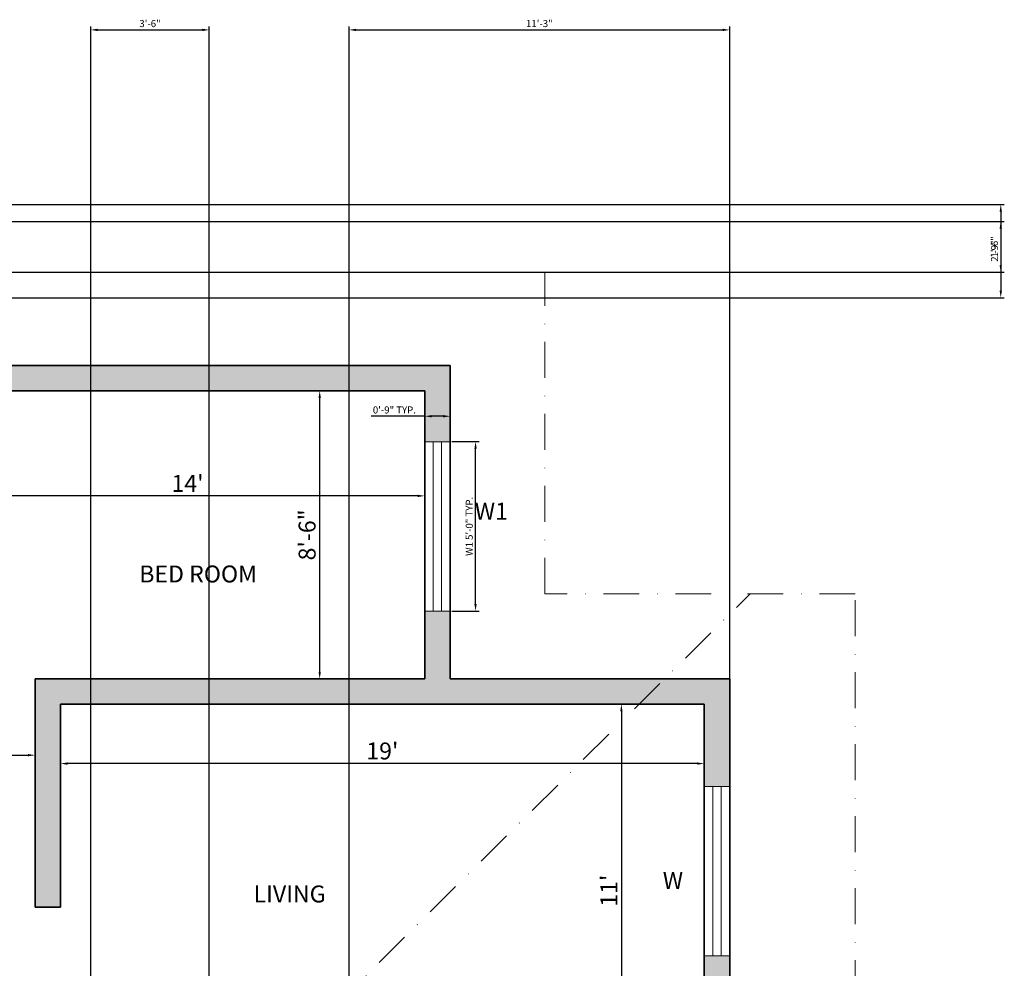
# Model space of a CAD drawing. Units: inches. Extents: x 4701 to 5398, y 2331 to 3130.
# Tile 3 of 3: x 5050 to 5398, y 2792 to 3128. Entities that reach past the tile are written whole.
import ezdxf

# ---------------------------------------------------------------- set-up
doc = ezdxf.new("R2010")
doc.units = ezdxf.units.IN
doc.linetypes.add('DASHDOT', pattern=[25.4, 12.7, -6.35, 0, -6.35])
for name, color, linetype, lineweight, true_color in [('A-ANNO-DIMS', 217, 'Continuous', 18, 0x93278f), ('A-GLAZ', 41, 'Continuous', 18, 0xf4ee51), ('A-WALL-PATT', 143, 'Continuous', 13, 0x7aafdf)]:
    doc.layers.add(name, color=color, linetype=linetype, lineweight=lineweight, true_color=true_color)
for name, color, linetype, lineweight in [('A-ANNO-TEXT', 7, 'Continuous', 18), ('A-AREA-IDEN', 7, 'Continuous', 25), ('A-ROOF-OVHD', 8, 'DASHDOT', 13), ('A-WALL', 7, 'Continuous', 35)]:
    doc.layers.add(name, color=color, linetype=linetype, lineweight=lineweight)
doc.styles.get("Standard").update_dxf_attribs({"font": 'arial.ttf'})
doc.dimstyles.new('ISO-25', dxfattribs={"dimtxt": 2.5, "dimasz": 2.5, "dimexe": 1.25, "dimexo": 0.625, "dimtad": 1, "dimlunit": 3, "dimtxsty": 'Standard', "dimcen": 2.5, "dimadec": 0, "dimazin": 0, "dimtfac": 1, "dimtmove": 0, "dimatfit": 3, "dimfxl": 1, "dimarcsym": 0})

# ---------------------------------------------------------------- blocks, each defined once
blk = doc.blocks.new('*D9')
at = {"layer": 'A-ANNO-DIMS', "color": 0, "lineweight": -2, "transparency": 16777216}
for p, q in [((5025.11, 2959.48), (5025.11, 2960.11)), ((5190.61, 2958.86), (5027.61, 2958.86)), ((5193.11, 2959.48), (5193.11, 2960.11))]:
    blk.add_line(p, q, dxfattribs=at)
at = {"layer": 'A-ANNO-DIMS', "color": 0, "transparency": 16777216}
for points in [[(5027.61, 2959.28), (5027.61, 2958.44), (5025.11, 2958.86)], [(5190.61, 2959.28), (5190.61, 2958.44), (5193.11, 2958.86)]]:
    blk.add_solid(points, dxfattribs=at)
at = {"layer": 'Defpoints', "color": 0, "transparency": 16777216}
for p in [(5025.11, 2958.86), (5025.11, 2958.86), (5193.11, 2958.86)]:
    blk.add_point(p, dxfattribs=at)
at = {"layer": 'A-ANNO-DIMS', "color": 0, "transparency": 16777216, "insert": (5109.11, 2962.5), "char_height": 6, "attachment_point": 5}
blk.add_mtext("14'", dxfattribs=at)
blk = doc.blocks.new('*D10')
at = {"layer": 'A-ANNO-DIMS', "color": 0, "lineweight": -2, "transparency": 16777216}
for p, q in [((5156.54, 2996.05), (5154.66, 2996.05)), ((5155.91, 2896.55), (5155.91, 2993.55)), ((5155.29, 2894.05), (5154.66, 2894.05))]:
    blk.add_line(p, q, dxfattribs=at)
at = {"layer": 'A-ANNO-DIMS', "color": 0, "transparency": 16777216}
for points in [[(5155.5, 2993.55), (5156.33, 2993.55), (5155.91, 2996.05)], [(5155.5, 2896.55), (5156.33, 2896.55), (5155.91, 2894.05)]]:
    blk.add_solid(points, dxfattribs=at)
at = {"layer": 'Defpoints', "color": 0, "transparency": 16777216}
for p in [(5155.91, 2996.05), (5157.16, 2996.05), (5155.91, 2894.05)]:
    blk.add_point(p, dxfattribs=at)
at = {"layer": 'A-ANNO-DIMS', "color": 0, "transparency": 16777216, "insert": (5152.23, 2945.05), "char_height": 6, "attachment_point": 5, "rotation": 90}
blk.add_mtext('8\'-6"', dxfattribs=at)
blk = doc.blocks.new('*D11')
at = {"layer": 'A-ANNO-DIMS', "color": 0, "lineweight": -2, "transparency": 16777216}
for p, q in [((5064.11, 2864.69), (5064.11, 2865.31)), ((5289.61, 2864.06), (5066.61, 2864.06)), ((5292.11, 2864.69), (5292.11, 2865.31))]:
    blk.add_line(p, q, dxfattribs=at)
at = {"layer": 'A-ANNO-DIMS', "color": 0, "transparency": 16777216}
for points in [[(5066.61, 2864.48), (5066.61, 2863.65), (5064.11, 2864.06)], [(5289.61, 2864.48), (5289.61, 2863.65), (5292.11, 2864.06)]]:
    blk.add_solid(points, dxfattribs=at)
at = {"layer": 'Defpoints', "color": 0, "transparency": 16777216}
for p in [(5064.11, 2864.06), (5064.11, 2864.06), (5292.11, 2864.06)]:
    blk.add_point(p, dxfattribs=at)
at = {"layer": 'A-ANNO-DIMS', "color": 0, "transparency": 16777216, "insert": (5178.11, 2867.75), "char_height": 6, "attachment_point": 5}
blk.add_mtext("19'", dxfattribs=at)
blk = doc.blocks.new('*D12')
at = {"layer": 'A-ANNO-DIMS', "color": 0, "lineweight": -2, "transparency": 16777216}
for p, q in [((5263.38, 2885.05), (5264, 2885.05)), ((5262.75, 2882.55), (5262.75, 2755.55)), ((5263.38, 2753.05), (5264, 2753.05))]:
    blk.add_line(p, q, dxfattribs=at)
at = {"layer": 'A-ANNO-DIMS', "color": 0, "transparency": 16777216}
for points in [[(5262.34, 2882.55), (5263.17, 2882.55), (5262.75, 2885.05)], [(5262.34, 2755.55), (5263.17, 2755.55), (5262.75, 2753.05)]]:
    blk.add_solid(points, dxfattribs=at)
at = {"layer": 'Defpoints', "color": 0, "transparency": 16777216}
for p in [(5262.75, 2885.05), (5262.75, 2753.05), (5262.75, 2753.05)]:
    blk.add_point(p, dxfattribs=at)
at = {"layer": 'A-ANNO-DIMS', "color": 0, "transparency": 16777216, "insert": (5259.12, 2819.05), "char_height": 6, "attachment_point": 5, "rotation": 90}
blk.add_mtext("11'", dxfattribs=at)
blk = doc.blocks.new('*D29')
at = {"layer": 'A-ANNO-DIMS', "color": 0, "lineweight": -2, "transparency": 16777216}
for p, q in [((4908.5, 2867.66), (4908.5, 2868.28)), ((4911, 2867.03), (5052.61, 2867.03)), ((5055.11, 2867.66), (5055.11, 2868.28))]:
    blk.add_line(p, q, dxfattribs=at)
at = {"layer": 'A-ANNO-DIMS', "color": 0, "transparency": 16777216}
for points in [[(4911, 2867.45), (4911, 2866.62), (4908.5, 2867.03)], [(5052.61, 2867.45), (5052.61, 2866.62), (5055.11, 2867.03)]]:
    blk.add_solid(points, dxfattribs=at)
at = {"layer": 'Defpoints', "color": 0, "transparency": 16777216}
for p in [(4908.5, 2867.03), (5055.11, 2867.03), (5055.11, 2867.03)]:
    blk.add_point(p, dxfattribs=at)
at = {"layer": 'A-ANNO-DIMS', "color": 0, "transparency": 16777216, "insert": (4981.8, 2868.94), "char_height": 2.5, "attachment_point": 5}
blk.add_mtext('12\'-2.61"', dxfattribs=at)
blk = doc.blocks.new('WIN-60IN')
for p, q in [((0, 9), (0, 0)), ((0, 9), (60, 9)), ((60, 9), (60, 0)), ((0, 6), (60, 6)), ((0, 3), (60, 3)), ((60, 0), (0, 0))]:
    blk.add_line(p, q)
blk = doc.blocks.new('*D37')
at = {"layer": 'A-ANNO-DIMS', "color": 0, "lineweight": -2, "transparency": 16777216}
for p, q in [((5202.73, 2978.07), (5212.36, 2978.07)), ((5211.11, 2920.57), (5211.11, 2975.57)), ((5202.73, 2918.07), (5212.36, 2918.07))]:
    blk.add_line(p, q, dxfattribs=at)
at = {"layer": 'A-ANNO-DIMS', "color": 0, "transparency": 16777216}
for points in [[(5210.69, 2975.57), (5211.53, 2975.57), (5211.11, 2978.07)], [(5210.69, 2920.57), (5211.53, 2920.57), (5211.11, 2918.07)]]:
    blk.add_solid(points, dxfattribs=at)
at = {"layer": 'Defpoints', "color": 0, "transparency": 16777216}
for p in [(5202.11, 2978.07), (5211.11, 2978.07), (5202.11, 2918.07)]:
    blk.add_point(p, dxfattribs=at)
at = {"layer": 'A-ANNO-DIMS', "color": 0, "transparency": 16777216, "insert": (5209.21, 2948.07), "char_height": 2.5, "attachment_point": 5, "rotation": 90}
blk.add_mtext('W1 5\'-0" TYP.', dxfattribs=at)
blk = doc.blocks.new('*D38')
at = {"layer": 'A-ANNO-DIMS', "color": 0, "lineweight": -2, "transparency": 16777216}
for p, q in [((5193.11, 2987.07), (5174.12, 2987.07)), ((5193.11, 2978.69), (5193.11, 2988.32)), ((5199.61, 2987.07), (5195.61, 2987.07)), ((5202.11, 2978.69), (5202.11, 2988.32))]:
    blk.add_line(p, q, dxfattribs=at)
at = {"layer": 'A-ANNO-DIMS', "color": 0, "transparency": 16777216}
for points in [[(5195.61, 2987.48), (5195.61, 2986.65), (5193.11, 2987.07)], [(5199.61, 2987.48), (5199.61, 2986.65), (5202.11, 2987.07)]]:
    blk.add_solid(points, dxfattribs=at)
at = {"layer": 'Defpoints', "color": 0, "transparency": 16777216}
for p in [(5193.11, 2987.07), (5193.11, 2978.07), (5202.11, 2978.07)]:
    blk.add_point(p, dxfattribs=at)
at = {"layer": 'A-ANNO-DIMS', "color": 0, "transparency": 16777216, "insert": (5182.37, 2988.97), "char_height": 2.5, "attachment_point": 5}
blk.add_mtext('0\'-9" TYP.', dxfattribs=at)
blk = doc.blocks.new('*D48')
at = {"layer": 'A-ANNO-DIMS', "color": 0, "lineweight": -2, "transparency": 16777216}
for p, q in [((5074.82, 2636.68), (5074.82, 3125.15)), ((5116.82, 2636.68), (5116.82, 3125.15)), ((5077.32, 3123.9), (5114.32, 3123.9))]:
    blk.add_line(p, q, dxfattribs=at)
at = {"layer": 'A-ANNO-DIMS', "color": 0, "transparency": 16777216}
for points in [[(5077.32, 3124.32), (5077.32, 3123.49), (5074.82, 3123.9)], [(5114.32, 3124.32), (5114.32, 3123.49), (5116.82, 3123.9)]]:
    blk.add_solid(points, dxfattribs=at)
at = {"layer": 'Defpoints', "color": 0, "transparency": 16777216}
for p in [(5116.82, 3123.9), (5074.82, 2636.05), (5116.82, 2636.05)]:
    blk.add_point(p, dxfattribs=at)
at = {"layer": 'A-ANNO-DIMS', "color": 0, "transparency": 16777216, "insert": (5095.82, 3125.81), "char_height": 2.5, "attachment_point": 5}
blk.add_mtext('3\'-6"', dxfattribs=at)
blk = doc.blocks.new('*D50')
at = {"layer": 'A-ANNO-DIMS', "color": 0, "lineweight": -2, "transparency": 16777216}
for p, q in [((5166.3, 2537.68), (5166.3, 3125.15)), ((5301.11, 2537.68), (5301.11, 3125.15)), ((5168.8, 3123.9), (5298.61, 3123.9))]:
    blk.add_line(p, q, dxfattribs=at)
at = {"layer": 'A-ANNO-DIMS', "color": 0, "transparency": 16777216}
for points in [[(5168.8, 3124.32), (5168.8, 3123.49), (5166.3, 3123.9)], [(5298.61, 3124.32), (5298.61, 3123.49), (5301.11, 3123.9)]]:
    blk.add_solid(points, dxfattribs=at)
at = {"layer": 'Defpoints', "color": 0, "transparency": 16777216}
for p in [(5301.11, 3123.9), (5166.3, 2537.05), (5301.11, 2537.05)]:
    blk.add_point(p, dxfattribs=at)
at = {"layer": 'A-ANNO-DIMS', "color": 0, "transparency": 16777216, "insert": (5233.71, 3125.81), "char_height": 2.5, "attachment_point": 5}
blk.add_mtext('11\'-3"', dxfattribs=at)
blk = doc.blocks.new('*D53')
at = {"layer": 'A-ANNO-DIMS', "color": 0, "lineweight": -2, "transparency": 16777216}
for p, q in [((4830.35, 3062.05), (5398.37, 3062.05)), ((5397.12, 3059.55), (5397.12, 3031.55)), ((4830.35, 3029.05), (5398.37, 3029.05))]:
    blk.add_line(p, q, dxfattribs=at)
at = {"layer": 'A-ANNO-DIMS', "color": 0, "transparency": 16777216}
for points in [[(5396.71, 3059.55), (5397.54, 3059.55), (5397.12, 3062.05)], [(5396.71, 3031.55), (5397.54, 3031.55), (5397.12, 3029.05)]]:
    blk.add_solid(points, dxfattribs=at)
at = {"layer": 'Defpoints', "color": 0, "transparency": 16777216}
for p in [(4829.72, 3062.05), (4829.72, 3029.05), (5397.12, 3029.05)]:
    blk.add_point(p, dxfattribs=at)
at = {"layer": 'A-ANNO-DIMS', "color": 0, "transparency": 16777216, "insert": (5395.22, 3045.55), "char_height": 2.5, "attachment_point": 5, "rotation": 90}
blk.add_mtext('2\'-9"', dxfattribs=at)
blk = doc.blocks.new('*D54')
at = {"layer": 'A-ANNO-DIMS', "color": 0, "lineweight": -2, "transparency": 16777216}
for p, q in [((4953.85, 3056.05), (5398.37, 3056.05)), ((5397.12, 3053.55), (5397.12, 3040.55)), ((4944.85, 3038.05), (5398.37, 3038.05))]:
    blk.add_line(p, q, dxfattribs=at)
at = {"layer": 'A-ANNO-DIMS', "color": 0, "transparency": 16777216}
for points in [[(5396.71, 3053.55), (5397.54, 3053.55), (5397.12, 3056.05)], [(5396.71, 3040.55), (5397.54, 3040.55), (5397.12, 3038.05)]]:
    blk.add_solid(points, dxfattribs=at)
at = {"layer": 'Defpoints', "color": 0, "transparency": 16777216}
for p in [(4953.22, 3056.05), (4944.22, 3038.05), (5397.12, 3038.05)]:
    blk.add_point(p, dxfattribs=at)
at = {"layer": 'A-ANNO-DIMS', "color": 0, "transparency": 16777216, "insert": (5395.22, 3047.05), "char_height": 2.5, "attachment_point": 5, "rotation": 90}
blk.add_mtext('1\'-6"', dxfattribs=at)

msp = doc.modelspace()

# ---------------------------------------------------------------- hatches: boundary and pattern name
at = {"layer": 'A-WALL-PATT'}
h = msp.add_hatch(color=256, dxfattribs=at)
h.dxf.hatch_style = 1
h.paths.add_polyline_path([(4829.723, 3062.054), (4820.723, 3062.054), (4772.223, 3062.054), (4772.223, 3050.208), (4781.223, 3050.208), (4781.223, 3053.054), (4820.723, 3053.054), (4820.723, 3050.208), (4829.723, 3050.208)])
h.paths.add_polyline_path([(4781.223, 3050.208), (4772.223, 3050.208), (4772.223, 3029.054), (4772.223, 2999.675), (4781.223, 2999.675), (4781.223, 3029.054)])
h.paths.add_polyline_path([(4781.223, 2918.054), (4864.223, 2918.054), (4899.497, 2918.054), (4899.497, 2845.832), (4908.497, 2845.832), (4908.497, 2918.054), (4908.497, 2927.054), (4893.11, 2927.054), (4893.11, 2954.328), (4884.11, 2954.328), (4884.11, 2927.054), (4864.223, 2927.054), (4781.223, 2927.054), (4781.223, 2951.675), (4772.223, 2951.675), (4772.223, 2918.054), (4772.223, 2884.79), (4781.223, 2884.79)])
h.paths.add_polyline_path([(4893.11, 3029.054), (4908.497, 3029.054), (4908.497, 3038.054), (4873.223, 3038.054), (4873.223, 3050.208), (4864.223, 3050.208), (4864.223, 3038.054), (4859.723, 3038.054), (4859.723, 3029.054), (4884.11, 3029.054), (4884.11, 2984.328), (4893.11, 2984.328)])
h.paths.add_polyline_path([(4873.223, 3078.054), (4878.497, 3078.054), (4878.497, 3087.054), (4864.223, 3087.054), (4864.223, 3050.208), (4873.223, 3050.208)])
h.paths.add_polyline_path([(4976.546, 3087.054), (4908.497, 3087.054), (4908.497, 3078.054), (4944.223, 3078.054), (4944.223, 3056.054), (4953.223, 3056.054), (4953.223, 3078.054), (4976.546, 3078.054)])
h.paths.add_polyline_path([(5044.223, 3087.054), (5000.546, 3087.054), (5000.546, 3078.054), (5035.223, 3078.054), (5035.223, 3038.054), (5044.223, 3038.054)])
h.paths.add_polyline_path([(5030.994, 3038.054), (5017.16, 3038.054), (4944.223, 3038.054), (4944.223, 3029.054), (5031.069, 3029.054)])
h.paths.add_polyline_path([(5044.223, 3038.054), (5035.223, 3038.054), (5030.994, 3038.054), (5031.069, 3029.054), (5044.223, 3029.054)])
h.paths.add_polyline_path([(5202.11, 3005.054), (5193.11, 3005.054), (5031.27, 3005.054), (5031.345, 2996.054), (5193.11, 2996.054), (5193.11, 2978.066), (5202.11, 2978.066), (5202.11, 2996.054)])
h.paths.add_polyline_path([(5031.27, 3005.054), (5025.11, 3005.054), (5016.11, 3005.054), (5016.11, 2903.054), (4962.304, 2903.054), (4962.304, 2894.054), (5025.11, 2894.054), (5025.11, 2996.054), (5031.345, 2996.054)])
h.paths.add_polyline_path([(5278.045, 2894.054), (5202.11, 2894.054), (5202.11, 2900.054), (5202.11, 2918.066), (5193.11, 2918.066), (5193.11, 2900.054), (5193.11, 2894.054), (5055.11, 2894.054), (5055.11, 2840.014), (5055.11, 2813.236), (5064.11, 2813.236), (5064.11, 2840.014), (5064.11, 2885.054), (5268.987, 2885.054)])
h.paths.add_polyline_path([(5301.11, 2894.054), (5278.045, 2894.054), (5268.987, 2885.054), (5292.11, 2885.054), (5292.11, 2855.934), (5301.11, 2855.934), (5301.11, 2885.054)])
h.paths.add_polyline_path([(5301.11, 2795.934), (5292.11, 2795.934), (5292.11, 2753.054), (5193.11, 2753.054), (5160.11, 2753.054), (5160.11, 2735.907), (5168.378, 2726.63), (5169.11, 2726.63), (5169.11, 2744.054), (5292.11, 2744.054), (5292.11, 2636.054), (5283.654, 2636.054), (5283.654, 2627.054), (5301.11, 2627.054)])
h.paths.add_polyline_path([(5160.11, 2735.907), (5160.11, 2726.63), (5168.378, 2726.63)], flags=17)
h.paths.add_polyline_path([(5064.11, 2746.827), (5055.11, 2746.827), (5055.11, 2727.054), (5033.595, 2727.054), (5033.671, 2718.054), (5055.11, 2718.054), (5055.11, 2627.054), (5055.11, 2546.054), (5035.539, 2546.054), (5035.539, 2537.054), (5064.11, 2537.054), (5064.11, 2627.054), (5074.819, 2627.054), (5074.819, 2636.054), (5064.11, 2636.054)])
h.paths.add_polyline_path([(5178.11, 2636.054), (5169.11, 2636.054), (5169.11, 2696.63), (5160.11, 2696.63), (5160.11, 2636.054), (5116.819, 2636.054), (5116.819, 2627.054), (5178.11, 2627.054)])
h.paths.add_polyline_path([(5235.654, 2636.054), (5220.11, 2636.054), (5220.11, 2627.054), (5235.654, 2627.054)], flags=17)
h.paths.add_polyline_path([(5033.595, 2727.054), (4994.096, 2727.054), (4994.096, 2718.054), (5033.671, 2718.054)])
h.paths.add_polyline_path([(4964.096, 2727.054), (4947.11, 2727.054), (4947.11, 2546.054), (4908.497, 2546.054), (4908.497, 2554.169), (4899.497, 2554.169), (4899.497, 2546.054), (4869.656, 2546.054), (4869.656, 2537.054), (4908.497, 2537.054), (4975.539, 2537.054), (4975.539, 2546.054), (4956.11, 2546.054), (4956.11, 2718.054), (4964.096, 2718.054)])
h.paths.add_polyline_path([(4827.656, 2546.054), (4781.223, 2546.054), (4781.223, 2577.475), (4772.223, 2577.475), (4772.223, 2537.054), (4827.656, 2537.054)])
h.paths.add_polyline_path([(4781.223, 2664.054), (4899.497, 2664.054), (4899.497, 2584.169), (4908.497, 2584.169), (4908.497, 2683.844), (4899.497, 2683.844), (4899.497, 2673.054), (4781.223, 2673.054), (4781.223, 2710.334), (4772.223, 2710.334), (4772.223, 2625.475), (4781.223, 2625.475)])
h.paths.add_polyline_path([(4908.497, 2815.832), (4899.497, 2815.832), (4899.497, 2800.054), (4864.223, 2800.054), (4781.223, 2800.054), (4781.223, 2836.79), (4772.223, 2836.79), (4772.223, 2758.334), (4781.223, 2758.334), (4781.223, 2791.054), (4899.497, 2791.054), (4899.497, 2713.844), (4908.497, 2713.844)])

# ---------------------------------------------------------------- linework, layer by layer
at = {"layer": 'A-GLAZ'}
msp.add_line((5193.11, 2918.066), (5193.11, 2918.066), dxfattribs=at)
at = {"layer": 'A-ROOF-OVHD'}
for p, q in [((5235.648, 3038.054), (5017.16, 3038.054)), ((5235.648, 2924.185), (5235.648, 3038.054)), ((5140.745, 2757.635), (5308.37, 2924.185)), ((5345.573, 2924.185), (5235.648, 2924.185)), ((5308.37, 2924.185), (5308.37, 2924.185)), ((5345.573, 2577.697), (5345.573, 2924.185))]:
    msp.add_line(p, q, dxfattribs=at)
at = {"layer": 'A-WALL'}
for p, q in [((5025.11, 3005.054), (5193.11, 3005.054)), ((5193.11, 3005.054), (5202.11, 3005.054)), ((5202.11, 3005.054), (5202.11, 2996.054)), ((5025.11, 2996.054), (5193.11, 2996.054)), ((5193.11, 2996.054), (5193.11, 2900.054)), ((5202.11, 2996.054), (5202.11, 2900.054)), ((5193.11, 2894.054), (5193.11, 2900.054)), ((5202.11, 2894.054), (5202.11, 2900.054)), ((5202.11, 2900.054), (5202.11, 2894.054)), ((5055.11, 2894.054), (5193.11, 2894.054)), ((5055.11, 2894.054), (5055.11, 2840.014)), ((5202.11, 2894.054), (5301.11, 2894.054)), ((5301.11, 2894.054), (5301.11, 2885.054)), ((5064.11, 2885.054), (5292.11, 2885.054)), ((5064.11, 2885.054), (5064.11, 2840.014)), ((5292.11, 2885.054), (5292.11, 2840.014)), ((5301.11, 2885.054), (5301.11, 2840.014)), ((5055.11, 2840.014), (5055.11, 2813.236)), ((5064.11, 2813.236), (5064.11, 2840.014)), ((5292.11, 2840.014), (5292.11, 2753.054)), ((5292.11, 2840.014), (5292.11, 2753.054)), ((5301.11, 2840.014), (5301.11, 2537.054)), ((5055.11, 2813.236), (5064.11, 2813.236))]:
    msp.add_line(p, q, dxfattribs=at)

# ---------------------------------------------------------------- block references
at = {"layer": 'A-GLAZ'}
for p, rotation in [((5202.11, 2918.066), 90.0000000000011), ((5301.11, 2795.935), 89.9999999999994)]:
    msp.add_blockref('WIN-60IN', p, dxfattribs=dict(at, rotation=rotation))

# ---------------------------------------------------------------- texts
at = {"layer": 'A-ANNO-TEXT', "char_height": 6, "attachment_point": 1}
for s, insert in [('W1', (5210.842, 2956.458)), ('W', (5277.421, 2825.675))]:
    msp.add_mtext_dynamic_manual_height_columns(s, width=53.21859, gutter_width=12.5, heights=[0], dxfattribs=dict(at, insert=insert))
at = {"layer": 'A-AREA-IDEN', "char_height": 6, "attachment_point": 1}
for s, insert in [(' BED ROOM', (5090.182, 2934.207)), (' LIVING', (5130.659, 2820.889))]:
    msp.add_mtext_dynamic_manual_height_columns(s, width=53.21859, gutter_width=12.5, heights=[0], dxfattribs=dict(at, insert=insert))

# ---------------------------------------------------------------- dimensions: what is measured, and where the dimension line sits
at = {"layer": 'A-ANNO-DIMS'}
for base, p1, p2, override, picture, middle in [((5116.819, 3123.904), (5074.819, 2636.054), (5116.819, 2636.054), {"dimdec": 1, "dimlfac": 1, "dimrnd": 0, "dimzin": 1, "dimdsep": 46, "dimlunit": 4, "dimfrac": 2}, '*D48', (5095.819, 3125.807)), ((5301.11, 3123.904), (5166.304, 2537.054), (5301.11, 2537.054), {"dimdec": 1, "dimlfac": 1, "dimrnd": 0, "dimzin": 1, "dimdsep": 46, "dimlunit": 4, "dimfrac": 2}, '*D50', (5233.707, 3125.807)), ((5025.11, 2958.859), (5193.11, 2958.859), (5025.11, 2958.859), {"dimtxt": 6, "dimclrd": 0, "dimclre": 0, "dimclrt": 0}, '*D9', (5109.11, 2962.496)), ((5055.11, 2867.034), (4908.497, 2867.034), (5055.11, 2867.034), {"dimclrd": 0, "dimclre": 0, "dimclrt": 0}, '*D29', (4981.804, 2868.936)), ((5064.11, 2864.064), (5292.11, 2864.064), (5064.11, 2864.064), {"dimtxt": 6, "dimclrd": 0, "dimclre": 0, "dimclrt": 0}, '*D11', (5178.11, 2867.753))]:
    dim = msp.add_linear_dim(base=base, p1=p1, p2=p2, dimstyle='ISO-25', override=override, dxfattribs=at)
    dim.commit()
    dim.dimension.update_dxf_attribs({"geometry": picture, "text_midpoint": middle})
for base, p1, p2, override, picture, middle in [((5397.124, 3029.054), (4829.723, 3062.054), (4829.723, 3029.054), {"dimdec": 1, "dimlfac": 1, "dimrnd": 0, "dimzin": 1, "dimdsep": 46, "dimlunit": 4, "dimfrac": 2}, '*D53', (5395.223, 3045.554)), ((5397.124, 3038.054), (4953.223, 3056.054), (4944.223, 3038.054), {"dimdec": 1, "dimlfac": 1, "dimrnd": 0, "dimzin": 1, "dimdsep": 46, "dimlunit": 4, "dimfrac": 2}, '*D54', (5395.223, 3047.054)), ((5262.754, 2753.054), (5262.754, 2885.054), (5262.754, 2753.054), {"dimtxt": 6, "dimclrd": 0, "dimclre": 0, "dimclrt": 0}, '*D12', (5259.117, 2819.054))]:
    dim = msp.add_linear_dim(base=base, p1=p1, p2=p2, angle=90, dimstyle='ISO-25', override=override, dxfattribs=at)
    dim.commit()
    dim.dimension.update_dxf_attribs({"geometry": picture, "text_midpoint": middle})
dim = msp.add_linear_dim(base=(5155.914, 2996.054), p1=(5155.914, 2894.054), p2=(5157.164, 2996.054), angle=90, dimstyle='ISO-25', override={"dimtxt": 6, "dimclrd": 0, "dimclre": 0, "dimclrt": 0}, dxfattribs=at)
dim.commit()
dim.dimension.update_dxf_attribs({"geometry": '*D10', "text_midpoint": (5155.914, 2945.054), "dimtype": 160})
for base, p1, p2, angle, text, picture, middle in [((5193.11, 2987.066), (5202.11, 2978.066), (5193.11, 2978.066), 180, '<> TYP.', '*D38', (5182.366, 2988.967)), ((5211.11, 2978.066), (5202.11, 2918.066), (5202.11, 2978.066), 90, 'W1 <> TYP.', '*D37', (5209.209, 2948.066))]:
    dim = msp.add_linear_dim(base=base, p1=p1, p2=p2, angle=angle, text=text, dimstyle='ISO-25', override={"dimdec": 1, "dimlfac": 1, "dimrnd": 0, "dimzin": 1, "dimdsep": 46, "dimlunit": 4, "dimfrac": 2}, dxfattribs=at)
    dim.commit()
    dim.dimension.update_dxf_attribs({"geometry": picture, "text_midpoint": middle})

doc.saveas('drawing.dxf')
